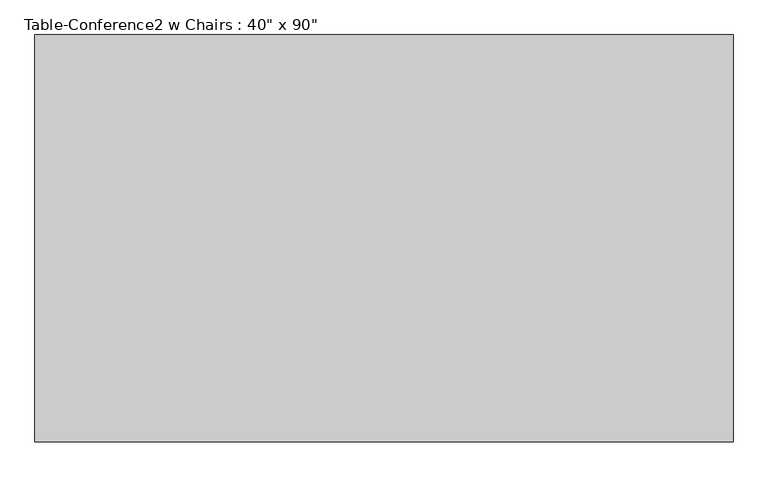
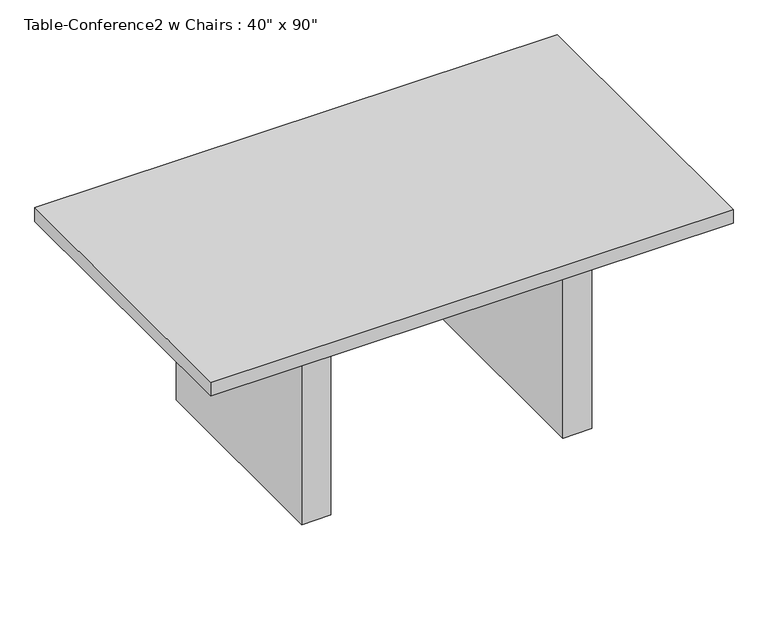
"""IFC4 building model written with IfcOpenShell, lengths in millimetres: furniture geometry."""

from ifc_helpers import new_model, si_unit, frame, origin, origin_with_axes, place, context, project, spatial, polyline, outline, extrude, source, transform, mapped, element, save


def furniture_65ba067b(model_context):
    return source(origin(), model_context, "Body", "SweptSolid", [
        extrude(outline(polyline([(914.4, -533.4), (-914.4, -533.4), (-914.4, 533.4), (914.4, 533.4), (914.4, -533.4)])), frame((0.0, 0.0, 711.2), z_axis=(0.0, 0.0, 1.0), x_axis=(1.0, 0.0, 0.0)), (0.0, 0.0, 1.0), 50.8),
        extrude(outline(polyline([(-406.4, -381.0), (-508.0, -381.0), (-508.0, 381.0), (-406.4, 381.0), (-406.4, -381.0)])), origin_with_axes(), (0.0, 0.0, 1.0), 711.2),
        extrude(outline(polyline([(508.0, -381.0), (406.4, -381.0), (406.4, 381.0), (508.0, 381.0), (508.0, -381.0)])), origin_with_axes(), (0.0, 0.0, 1.0), 711.2),
        extrude(outline(polyline([(406.4, 381.0), (406.4, 342.9), (-406.4, 342.9), (-406.4, 381.0), (406.4, 381.0)])), frame((0.0, 0.0, 609.6), z_axis=(0.0, 0.0, 1.0), x_axis=(1.0, 0.0, 0.0)), (0.0, 0.0, 1.0), 101.6),
        extrude(outline(polyline([(406.4, -381.0), (-406.4, -381.0), (-406.4, -342.9), (406.4, -342.9), (406.4, -381.0)])), frame((0.0, 0.0, 609.6), z_axis=(0.0, 0.0, 1.0), x_axis=(1.0, 0.0, 0.0)), (0.0, 0.0, 1.0), 101.6),
    ])


if __name__ == "__main__":
    model = new_model("IFC4")
    model_context = context("Model", 3, world=origin())
    ifc_project = project(units=[si_unit("LENGTHUNIT", "METRE", prefix="MILLI")], contexts=[model_context])
    site = spatial("IfcSite", under=ifc_project)
    building = spatial("IfcBuilding", under=site)
    placement = place(None, origin())
    furniture_shape = furniture_65ba067b(model_context)
    element("IfcFurniture", 1, ObjectType="Table-Conference2 w Chairs : 40\" x 90\"", at=placement, inside=building, context=model_context, shape_type="MappedRepresentation", body=[
        mapped(furniture_shape, transform((0.0, 0.0, 0.0), x_axis=(1.0, 0.0, 0.0), y_axis=(0.0, 1.0, 0.0), z_axis=(0.0, 0.0, 1.0))),
    ])
    save(model, "model.ifc")

# Revit data of these elements
# Type "Table-Conference2 w Chairs : 40\" x 90\""
#   Assembly Code = "E2020200"
#   Description = "Seating 6-8"
#   Height = 2' - 6"
#   Length = 6' - 0"
#   Width = 3' - 6"
#   Number Of Chairs One Side = 2
#   Number Of Chairs = 6
#   Material = Wood - Cherry
#   Default Elevation = 0
# Element 1 (IfcFurniture, "Table-Conference2 w Chairs : 40\" x 90\"")
#   Materials on its faces: "Wood - Cherry"
# Materials
#   "Wood - Cherry": colour RGB 151 75 0, transparency 0
